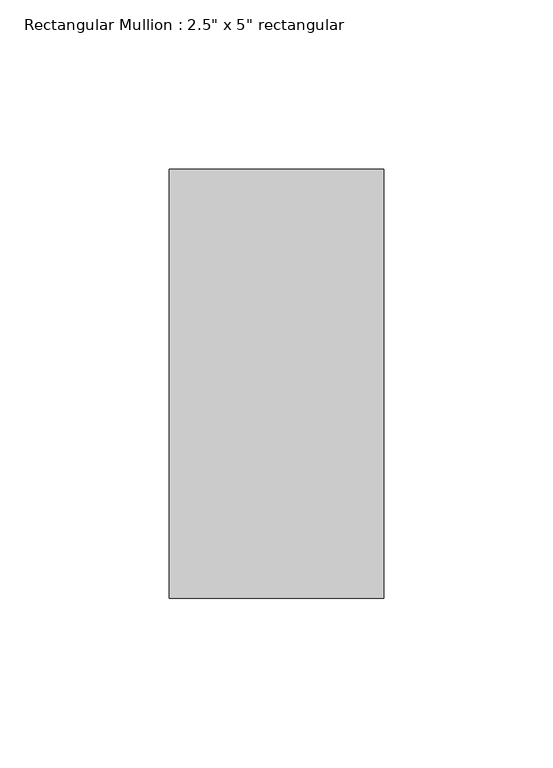
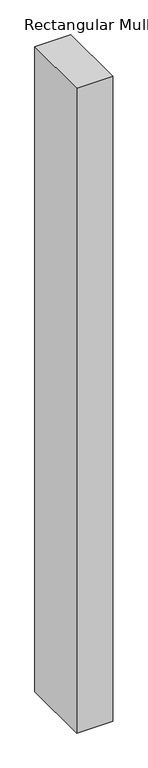
"""IFC4 building model written with IfcOpenShell, lengths in millimetres: member geometry."""

from ifc_helpers import new_model, si_unit, frame, origin, place, context, project, spatial, polyline, outline, extrude, source, transform, mapped, element, save


def member_e9c7f4a4(model_context):
    return source(origin(), model_context, "Body", "SweptSolid", [
        extrude(outline(polyline([(0.0, 63.5), (0.0, -63.5), (-63.5, -63.5), (-63.5, 63.5), (0.0, 63.5)])), frame((0.0, 0.0, -1200.15), z_axis=(0.0, 0.0, 1.0), x_axis=(1.0, 0.0, 0.0)), (0.0, 0.0, 1.0), 1200.15),
    ])


if __name__ == "__main__":
    model = new_model("IFC4")
    model_context = context("Model", 3, world=origin())
    ifc_project = project(units=[si_unit("LENGTHUNIT", "METRE", prefix="MILLI")], contexts=[model_context])
    site = spatial("IfcSite", under=ifc_project)
    building = spatial("IfcBuilding", under=site)
    placement = place(None, origin())
    member_shape = member_e9c7f4a4(model_context)
    element("IfcMember", 1, ObjectType="Rectangular Mullion : 2.5\" x 5\" rectangular", at=placement, inside=building, context=model_context, shape_type="MappedRepresentation", body=[
        mapped(member_shape, transform((0.0, 0.0, 0.0), x_axis=(1.0, 0.0, 0.0), y_axis=(0.0, 1.0, 0.0), z_axis=(0.0, 0.0, 1.0))),
    ])
    save(model, "model.ifc")

# Revit data of these elements
# Type "Rectangular Mullion : 2.5\" x 5\" rectangular"
#   built-in parameter 1007304 = 0.416667 (stored number, unit not read)
#   built-in parameter 1007301 = 0.104167 (stored number, unit not read)
#   built-in parameter 1007300 = 0.104167 (stored number, unit not read)
# Element 1 (IfcMember, "Rectangular Mullion : 2.5\" x 5\" rectangular")
#   Materials on its faces: "Aluminum"
# Materials
#   "Aluminum": class "Metal", colour RGB 247 247 247, transparency 0, Description = "Aluminum 6061", Cost = 0
